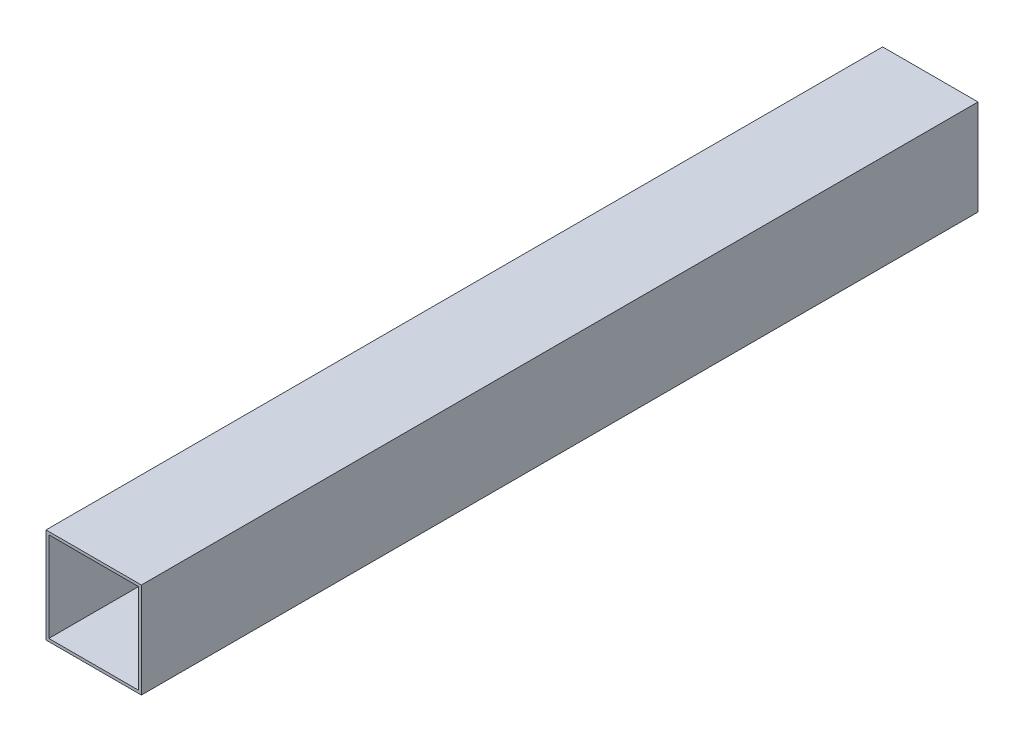
SolidWorks part; units mm, degrees
material "Plain Carbon Steel"
ref_plane "Front Plane" through (0, 0, 0) normal (0, 0, 1) x (1, 0, 0)
ref_plane "Top Plane" through (0, 0, 0) normal (0, 1, 0) x (1, 0, 0)
ref_plane "Right Plane" through (0, 0, 0) normal (1, 0, 0) x (0, 0, -1)
sketch "Tube Profile 8x8 Square" plane through (0, 0, 0) normal (0, 0, 1) x (1, 0, 0)
  line L1 (-101.6, 101.6) -> (101.6, 101.6)
  line L2 (-101.6, 101.6) -> (-101.6, -101.6)
  line L3 (-101.6, -101.6) -> (101.6, -101.6)
  line L4 (101.6, 101.6) -> (101.6, -101.6)
  line L5 (-101.6, 101.6) -> (101.6, -101.6) construction
  line L6 (-101.6, -101.6) -> (101.6, 101.6) construction
  point P0 (0, 0)
  dimension "D1" = 203.2
  dimension "D2" = 203.2
extrude "Square Tube 8.5x8.5x0.25 Wall" add sketch "Tube Profile 8x8 Square" along normal blind 1893.8875 thin contours L2 L3 L4 L1 thin type one direction wall 6.35
